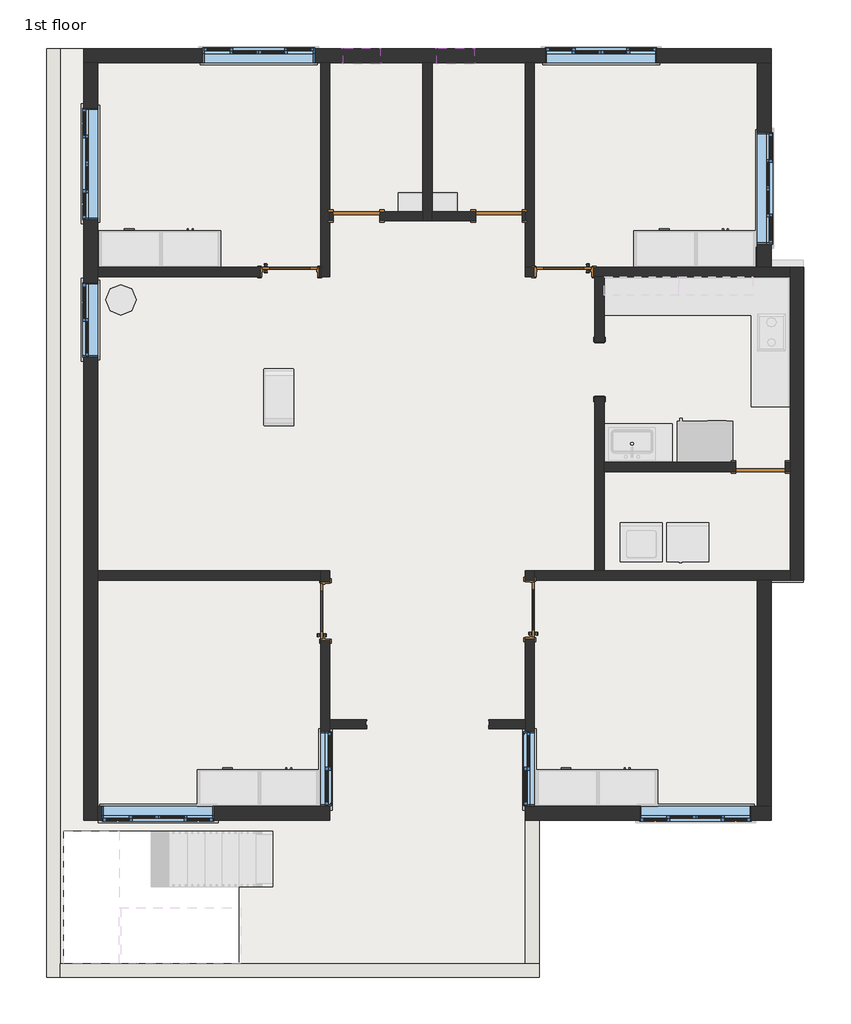
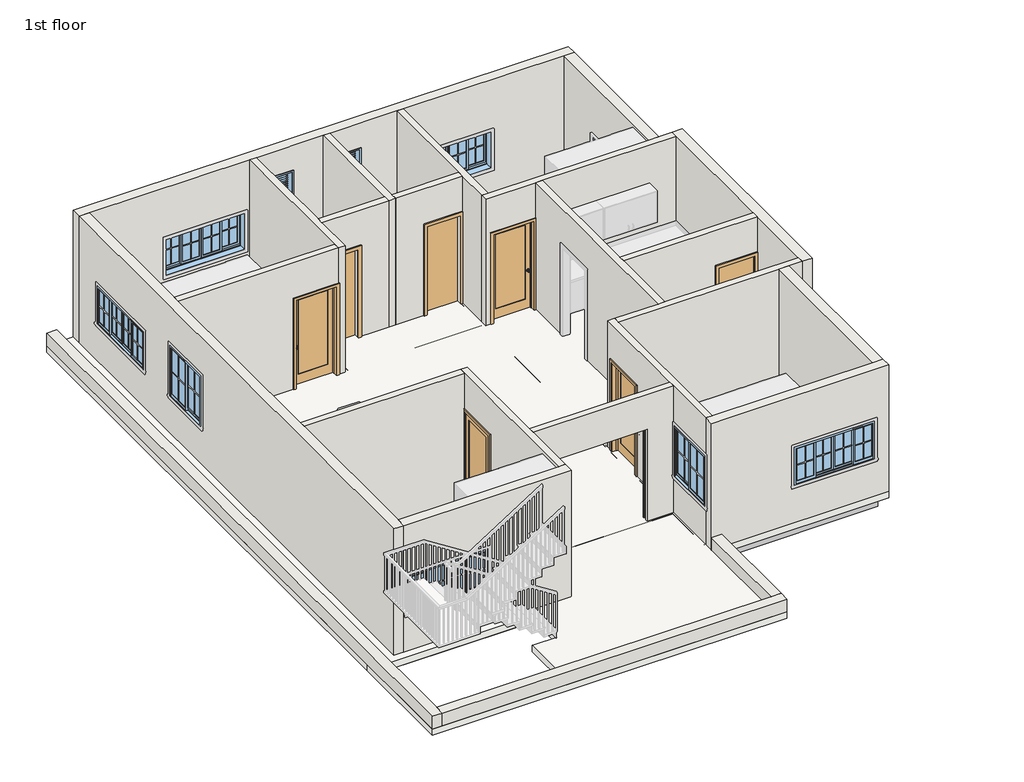
# One storey, part 1 of 4: 24 walls, 11 windows, 7 beams, 7 doors, 1 slab.
# Revit data of these elements (continued)
# Element 45 (IfcWindow, "Window-Sliding-Four : 72\" x 36\"") (continued)
#   Interior Wall Closure = 0' - 2 3/4"
#   Frame Extension = 0' - 0 1/4"
#   Exterior Wall Closure = 0' - 1 1/4"
#   Interior Trim Visibility = yes
#   Indicator Visibility = yes
#   Exterior Trim Visibility = yes
#   Phase Created = New Construction
#   Materials on its faces: "Wood - Stained", "Glass", "Clad - White"
# Element 46 (IfcWindow, "Window-Sliding-Four : 72\" x 36\"")
#   Mark = "18"
#   Window Inset = 0' - 0"
#   Interior Wall Closure = 0' - 2 3/4"
#   Frame Extension = 0' - 0 1/4"
#   Exterior Wall Closure = 0' - 1 1/4"
#   Interior Trim Visibility = yes
#   Indicator Visibility = yes
#   Exterior Trim Visibility = yes
#   Phase Created = New Construction
#   Materials on its faces: "Wood - Stained", "Glass", "Clad - White"
# Element 47 (IfcWindow, "Window-Sliding-Four : 72\" x 36\"")
#   Mark = "19"
#   Window Inset = 0' - 0"
#   Interior Wall Closure = 0' - 2 3/4"
#   Frame Extension = 0' - 0 1/4"
#   Exterior Wall Closure = 0' - 1 1/4"
#   Interior Trim Visibility = yes
#   Indicator Visibility = yes
#   Exterior Trim Visibility = yes
#   Phase Created = New Construction
#   Materials on its faces: "Wood - Stained", "Glass", "Clad - White"
# Element 48 (IfcWindow, "Window-Sliding-Four : 72\" x 36\"")
#   Mark = "20"
#   Window Inset = 0' - 0"
#   Interior Wall Closure = 0' - 2 3/4"
#   Frame Extension = 0' - 0 1/4"
#   Exterior Wall Closure = 0' - 1 1/4"
#   Interior Trim Visibility = yes
#   Indicator Visibility = yes
#   Exterior Trim Visibility = yes
#   Phase Created = New Construction
#   Materials on its faces: "Wood - Stained", "Glass", "Clad - White"
# Element 49 (IfcWindow, "Window-Sliding-Four : 72\" x 36\"")
#   Mark = "24"
#   Window Inset = 0' - 0"
#   Interior Wall Closure = 0' - 2 3/4"
#   Frame Extension = 0' - 0 1/4"
#   Exterior Wall Closure = 0' - 1 1/4"
#   Interior Trim Visibility = yes
#   Indicator Visibility = yes
#   Exterior Trim Visibility = yes
#   Phase Created = New Construction
#   Materials on its faces: "Wood - Stained", "Glass", "Clad - White"
# Element 50 (IfcWindow, "Window-Sliding-Four : 72\" x 36\"")
#   Mark = "25"
#   Window Inset = 0' - 0"
#   Interior Wall Closure = 0' - 2 3/4"
#   Frame Extension = 0' - 0 1/4"
#   Exterior Wall Closure = 0' - 1 1/4"
#   Interior Trim Visibility = yes
#   Indicator Visibility = yes
#   Exterior Trim Visibility = yes
#   Phase Created = New Construction
#   Materials on its faces: "Wood - Stained", "Glass", "Clad - White"
# Materials
#   "Concrete, Cast-in-Place gray": class "Concrete", colour RGB 192 192 192, transparency 0, Description = "Cast-in-place concrete", Cost = 0
#   "Cherry": class "Wood", colour RGB 226 177 128, transparency 0, Description = "Prunus Serotina", Cost = 0
#   "Aluminum": class "Metal", colour RGB 247 247 247, transparency 0, Description = "Aluminum 6061", Cost = 0
#   "Door - Panel": class "Wood", colour RGB 210 159 95, transparency 0, Cost = 0
#   "Door - Frame": colour RGB 118 70 51, transparency 0, Cost = 0
#   "Birch": class "Wood", colour RGB 224 178 126, transparency 0, Description = "Betula Alleghaniensis", Cost = 0
#   "Wood - Stained": class "Wood", colour RGB 224 178 126, transparency 0, Cost = 0
#   "Glass": class "Glass", colour RGB 0 128 192, transparency 0.75, Description = "Soda Lime Glass", Cost = 0
#   "Clad - White": class "Wood", colour RGB 242 242 238, transparency 0, Cost = 0
#   "Default Floor": colour RGB 128 128 128, transparency 0, Cost = 0
#   "Default Wall": colour RGB 128 128 128, transparency 0, Cost = 0
